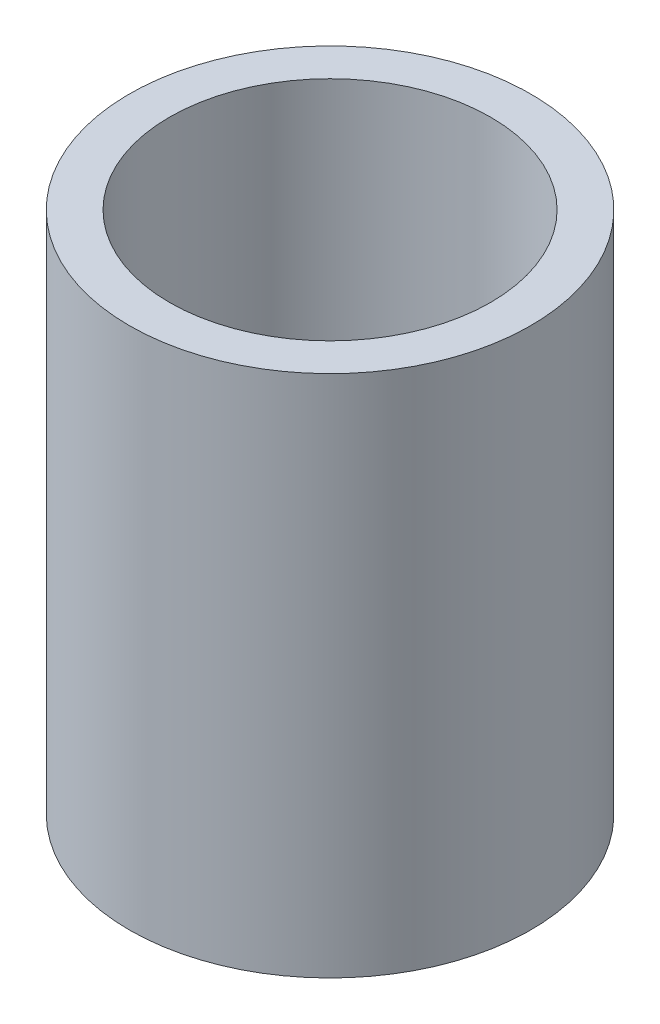
from build123d import *

# Parameters (mm, degrees)
TUBE_PROFILE_125_100_R   = 62.5
TUBE_PROFILE_125_100_R_2 = 50
SPACER_TUBE_L163_DEPTH   = 81.5


with BuildPart() as part:
    # Tube Profile Ø125-Ø100 → Spacer Tube L163 (new, symmetric)
    with BuildSketch(Plane(origin=(0, 0, 0), x_dir=(1, 0, 0), z_dir=(0, 1, 0))):
        with Locations(Location((0, 0, 0), (0, 0, 270))):
            Circle(TUBE_PROFILE_125_100_R)
        with Locations(Location((0, 0, 0), (0, 0, 270))):
            Circle(TUBE_PROFILE_125_100_R_2, mode=Mode.SUBTRACT)
    extrude(amount=SPACER_TUBE_L163_DEPTH, both=True)


solid = part.part
